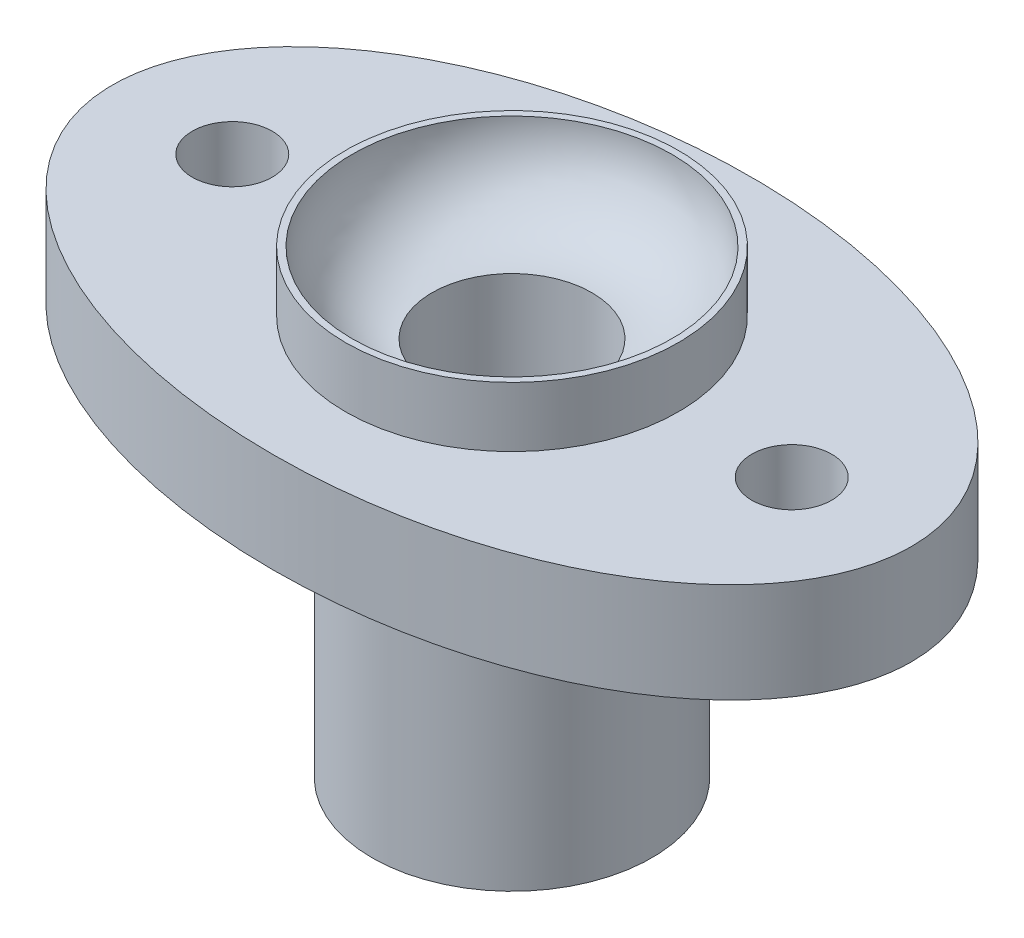
ISO-10303-21;
HEADER;
FILE_DESCRIPTION(('STEP AP214'),'2;1');
FILE_NAME('part.step','',(''),(''),'','','');
FILE_SCHEMA(('AUTOMOTIVE_DESIGN { 1 0 10303 214 1 1 1 1 }'));
ENDSEC;
DATA;
#1=APPLICATION_CONTEXT('core data for automotive mechanical design processes');
#2=APPLICATION_PROTOCOL_DEFINITION('international standard','automotive_design',2000,#1);
#3=PRODUCT_CONTEXT('',#1,'mechanical');
#4=PRODUCT('Part','Part','',(#3));
#5=PRODUCT_RELATED_PRODUCT_CATEGORY('part','',(#4));
#6=PRODUCT_DEFINITION_FORMATION('','',#4);
#7=PRODUCT_DEFINITION_CONTEXT('part definition',#1,'design');
#8=PRODUCT_DEFINITION('design','',#6,#7);
#9=PRODUCT_DEFINITION_SHAPE('','',#8);
#10=(LENGTH_UNIT() NAMED_UNIT(*) SI_UNIT(.MILLI.,.METRE.));
#11=(NAMED_UNIT(*) PLANE_ANGLE_UNIT() SI_UNIT($,.RADIAN.));
#12=(NAMED_UNIT(*) SI_UNIT($,.STERADIAN.) SOLID_ANGLE_UNIT());
#13=UNCERTAINTY_MEASURE_WITH_UNIT(LENGTH_MEASURE(1.E-05),#10,'distance_accuracy_value','');
#14=(GEOMETRIC_REPRESENTATION_CONTEXT(3) GLOBAL_UNCERTAINTY_ASSIGNED_CONTEXT((#13)) GLOBAL_UNIT_ASSIGNED_CONTEXT((#10,
#11,#12)) REPRESENTATION_CONTEXT('',''));
#15=CARTESIAN_POINT('',(0.,0.,0.));
#16=DIRECTION('',(0.,0.,1.));
#17=DIRECTION('',(1.,0.,0.));
#18=AXIS2_PLACEMENT_3D('',#15,#16,#17);
#19=CARTESIAN_POINT('',(0.,45.,0.));
#20=DIRECTION('',(0.,-1.,0.));
#21=DIRECTION('',(0.,0.,-1.));
#22=AXIS2_PLACEMENT_3D('',#19,#20,#21);
#23=CYLINDRICAL_SURFACE('',#22,21.);
#24=CARTESIAN_POINT('',(0.,45.,0.));
#25=DIRECTION('',(0.,1.,0.));
#26=DIRECTION('',(0.,0.,1.));
#27=AXIS2_PLACEMENT_3D('',#24,#25,#26);
#28=CIRCLE('',#27,21.);
#29=CARTESIAN_POINT('',(0.,45.,-21.));
#30=VERTEX_POINT('',#29);
#31=EDGE_CURVE('E10',#30,#30,#28,.T.);
#32=CARTESIAN_POINT('',(0.,0.,0.));
#33=DIRECTION('',(0.,-1.,0.));
#34=DIRECTION('',(0.,0.,-1.));
#35=AXIS2_PLACEMENT_3D('',#32,#33,#34);
#36=CIRCLE('',#35,21.);
#37=CARTESIAN_POINT('',(0.,0.,-21.));
#38=VERTEX_POINT('',#37);
#39=EDGE_CURVE('E73',#38,#38,#36,.T.);
#40=CARTESIAN_POINT('',(0.,45.,-21.));
#41=CARTESIAN_POINT('',(0.,44.53125,-21.));
#42=CARTESIAN_POINT('',(0.,44.0625,-21.));
#43=CARTESIAN_POINT('',(0.,43.125,-21.));
#44=CARTESIAN_POINT('',(0.,42.65625,-21.));
#45=CARTESIAN_POINT('',(0.,41.71875,-21.));
#46=CARTESIAN_POINT('',(0.,41.25,-21.));
#47=CARTESIAN_POINT('',(0.,40.3125,-21.));
#48=CARTESIAN_POINT('',(0.,39.84375,-21.));
#49=CARTESIAN_POINT('',(0.,38.90625,-21.));
#50=CARTESIAN_POINT('',(0.,38.4375,-21.));
#51=CARTESIAN_POINT('',(0.,37.5,-21.));
#52=CARTESIAN_POINT('',(0.,37.03125,-21.));
#53=CARTESIAN_POINT('',(0.,36.09375,-21.));
#54=CARTESIAN_POINT('',(0.,35.625,-21.));
#55=CARTESIAN_POINT('',(0.,34.6875,-21.));
#56=CARTESIAN_POINT('',(0.,34.21875,-21.));
#57=CARTESIAN_POINT('',(0.,33.28125,-21.));
#58=CARTESIAN_POINT('',(0.,32.8125,-21.));
#59=CARTESIAN_POINT('',(0.,31.875,-21.));
#60=CARTESIAN_POINT('',(0.,31.40625,-21.));
#61=CARTESIAN_POINT('',(0.,30.46875,-21.));
#62=CARTESIAN_POINT('',(0.,30.,-21.));
#63=CARTESIAN_POINT('',(0.,29.0625,-21.));
#64=CARTESIAN_POINT('',(0.,28.59375,-21.));
#65=CARTESIAN_POINT('',(0.,27.65625,-21.));
#66=CARTESIAN_POINT('',(0.,27.1875,-21.));
#67=CARTESIAN_POINT('',(0.,26.25,-21.));
#68=CARTESIAN_POINT('',(0.,25.78125,-21.));
#69=CARTESIAN_POINT('',(0.,24.84375,-21.));
#70=CARTESIAN_POINT('',(0.,24.375,-21.));
#71=CARTESIAN_POINT('',(0.,23.4375,-21.));
#72=CARTESIAN_POINT('',(0.,22.96875,-21.));
#73=CARTESIAN_POINT('',(0.,22.03125,-21.));
#74=CARTESIAN_POINT('',(0.,21.5625,-21.));
#75=CARTESIAN_POINT('',(0.,20.625,-21.));
#76=CARTESIAN_POINT('',(0.,20.15625,-21.));
#77=CARTESIAN_POINT('',(0.,19.21875,-21.));
#78=CARTESIAN_POINT('',(0.,18.75,-21.));
#79=CARTESIAN_POINT('',(0.,17.8125,-21.));
#80=CARTESIAN_POINT('',(0.,17.34375,-21.));
#81=CARTESIAN_POINT('',(0.,16.40625,-21.));
#82=CARTESIAN_POINT('',(0.,15.9375,-21.));
#83=CARTESIAN_POINT('',(0.,15.,-21.));
#84=CARTESIAN_POINT('',(0.,14.53125,-21.));
#85=CARTESIAN_POINT('',(0.,13.59375,-21.));
#86=CARTESIAN_POINT('',(0.,13.125,-21.));
#87=CARTESIAN_POINT('',(0.,12.1875,-21.));
#88=CARTESIAN_POINT('',(0.,11.71875,-21.));
#89=CARTESIAN_POINT('',(0.,10.78125,-21.));
#90=CARTESIAN_POINT('',(0.,10.3125,-21.));
#91=CARTESIAN_POINT('',(0.,9.37500000000003,-21.));
#92=CARTESIAN_POINT('',(0.,8.90625000000003,-21.));
#93=CARTESIAN_POINT('',(0.,7.96875000000003,-21.));
#94=CARTESIAN_POINT('',(0.,7.50000000000003,-21.));
#95=CARTESIAN_POINT('',(0.,6.56250000000003,-21.));
#96=CARTESIAN_POINT('',(0.,6.09375000000003,-21.));
#97=CARTESIAN_POINT('',(0.,5.15625000000003,-21.));
#98=CARTESIAN_POINT('',(0.,4.68750000000003,-21.));
#99=CARTESIAN_POINT('',(0.,3.75000000000003,-21.));
#100=CARTESIAN_POINT('',(0.,3.28125000000003,-21.));
#101=CARTESIAN_POINT('',(0.,2.34375000000003,-21.));
#102=CARTESIAN_POINT('',(0.,1.87500000000003,-21.));
#103=CARTESIAN_POINT('',(0.,0.937500000000033,-21.));
#104=CARTESIAN_POINT('',(0.,0.468750000000034,-21.));
#105=CARTESIAN_POINT('',(0.,0.,-21.));
#106=B_SPLINE_CURVE_WITH_KNOTS('',3,(#40,#41,#42,#43,#44,#45,#46,#47,#48,#49,#50,#51,#52,#53,
#54,#55,#56,#57,#58,#59,#60,#61,#62,#63,#64,#65,#66,#67,#68,#69,#70,#71,#72,#73,#74,#75,#76,#77,
#78,#79,#80,#81,#82,#83,#84,#85,#86,#87,#88,#89,#90,#91,#92,#93,#94,#95,#96,#97,#98,#99,#100,
#101,#102,#103,#104,#105),.UNSPECIFIED.,.F.,.F.,(4,2,2,2,2,2,2,2,2,2,2,2,2,2,2,2,2,2,2,2,2,2,2,
2,2,2,2,2,2,2,2,2,4),(0.,1.40625,2.8125,4.21875,5.625,7.03125,8.43749999999999,9.84375,11.25,
12.65625,14.0625,15.46875,16.875,18.28125,19.6875,21.09375,22.5,23.90625,25.3125,26.71875,
28.125,29.53125,30.9375,32.34375,33.75,35.15625,36.5625,37.96875,39.375,40.78125,42.1875,
43.59375,45.),.UNSPECIFIED.);
#107=EDGE_CURVE('BSEAM40',#30,#38,#106,.T.);
#108=ORIENTED_EDGE('',*,*,#31,.F.);
#109=ORIENTED_EDGE('',*,*,#39,.F.);
#110=ORIENTED_EDGE('',*,*,#107,.T.);
#111=ORIENTED_EDGE('',*,*,#107,.F.);
#112=EDGE_LOOP('',(#108,#110,#109,#111));
#113=FACE_BOUND('',#112,.T.);
#114=ADVANCED_FACE('F40',(#113),#23,.T.);
#115=CARTESIAN_POINT('',(0.,60.,0.));
#116=DIRECTION('',(0.,1.,0.));
#117=DIRECTION('',(1.,0.,0.));
#118=AXIS2_PLACEMENT_3D('',#115,#116,#117);
#119=ELLIPSE('',#118,60.,36.);
#120=DIRECTION('',(0.,-1.,0.));
#121=VECTOR('',#120,1.);
#122=SURFACE_OF_LINEAR_EXTRUSION('',#119,#121);
#123=CARTESIAN_POINT('',(60.,60.,0.));
#124=VERTEX_POINT('',#123);
#125=EDGE_CURVE('E42',#124,#124,#119,.T.);
#126=ORIENTED_EDGE('',*,*,#125,.F.);
#127=EDGE_LOOP('',(#126));
#128=FACE_BOUND('',#127,.T.);
#129=CARTESIAN_POINT('',(0.,45.,0.));
#130=DIRECTION('',(0.,1.,0.));
#131=DIRECTION('',(1.,0.,0.));
#132=AXIS2_PLACEMENT_3D('',#129,#130,#131);
#133=ELLIPSE('',#132,60.,36.);
#134=CARTESIAN_POINT('',(60.,45.,0.));
#135=VERTEX_POINT('',#134);
#136=EDGE_CURVE('E47',#135,#135,#133,.T.);
#137=ORIENTED_EDGE('',*,*,#136,.T.);
#138=EDGE_LOOP('',(#137));
#139=FACE_BOUND('',#138,.T.);
#140=ADVANCED_FACE('F84',(#128,#139),#122,.F.);
#141=CARTESIAN_POINT('',(0.,60.,0.));
#142=DIRECTION('',(0.,1.,0.));
#143=DIRECTION('',(0.,0.,1.));
#144=AXIS2_PLACEMENT_3D('',#141,#142,#143);
#145=PLANE('',#144);
#146=CARTESIAN_POINT('',(-42.,60.,0.));
#147=DIRECTION('',(0.,1.,0.));
#148=DIRECTION('',(0.,0.,1.));
#149=AXIS2_PLACEMENT_3D('',#146,#147,#148);
#150=CIRCLE('',#149,6.00000000000001);
#151=CARTESIAN_POINT('',(-42.,60.,6.00000000000001));
#152=VERTEX_POINT('',#151);
#153=EDGE_CURVE('E53',#152,#152,#150,.T.);
#154=ORIENTED_EDGE('',*,*,#153,.F.);
#155=EDGE_LOOP('',(#154));
#156=FACE_BOUND('',#155,.T.);
#157=CARTESIAN_POINT('',(42.,60.,0.));
#158=DIRECTION('',(0.,1.,0.));
#159=DIRECTION('',(0.,0.,1.));
#160=AXIS2_PLACEMENT_3D('',#157,#158,#159);
#161=CIRCLE('',#160,6.00000000000001);
#162=CARTESIAN_POINT('',(42.,60.,6.00000000000001));
#163=VERTEX_POINT('',#162);
#164=EDGE_CURVE('E58',#163,#163,#161,.T.);
#165=ORIENTED_EDGE('',*,*,#164,.F.);
#166=EDGE_LOOP('',(#165));
#167=FACE_BOUND('',#166,.T.);
#168=CARTESIAN_POINT('',(0.,60.,0.));
#169=DIRECTION('',(0.,1.,0.));
#170=DIRECTION('',(0.,0.,1.));
#171=AXIS2_PLACEMENT_3D('',#168,#169,#170);
#172=CIRCLE('',#171,25.);
#173=CARTESIAN_POINT('',(0.,60.,25.));
#174=VERTEX_POINT('',#173);
#175=EDGE_CURVE('E78',#174,#174,#172,.T.);
#176=ORIENTED_EDGE('',*,*,#175,.F.);
#177=EDGE_LOOP('',(#176));
#178=FACE_BOUND('',#177,.T.);
#179=ORIENTED_EDGE('',*,*,#125,.T.);
#180=EDGE_LOOP('',(#179));
#181=FACE_BOUND('',#180,.T.);
#182=ADVANCED_FACE('F87',(#156,#167,#178,#181),#145,.T.);
#183=CARTESIAN_POINT('',(0.,45.,0.));
#184=DIRECTION('',(0.,1.,0.));
#185=DIRECTION('',(0.,0.,1.));
#186=AXIS2_PLACEMENT_3D('',#183,#184,#185);
#187=PLANE('',#186);
#188=CARTESIAN_POINT('',(-42.,45.,0.));
#189=DIRECTION('',(0.,1.,0.));
#190=DIRECTION('',(0.,0.,1.));
#191=AXIS2_PLACEMENT_3D('',#188,#189,#190);
#192=CIRCLE('',#191,6.00000000000001);
#193=CARTESIAN_POINT('',(-42.,45.,6.00000000000001));
#194=VERTEX_POINT('',#193);
#195=EDGE_CURVE('E37',#194,#194,#192,.T.);
#196=ORIENTED_EDGE('',*,*,#195,.T.);
#197=EDGE_LOOP('',(#196));
#198=FACE_BOUND('',#197,.T.);
#199=CARTESIAN_POINT('',(42.,45.,0.));
#200=DIRECTION('',(0.,1.,0.));
#201=DIRECTION('',(0.,0.,1.));
#202=AXIS2_PLACEMENT_3D('',#199,#200,#201);
#203=CIRCLE('',#202,6.00000000000001);
#204=CARTESIAN_POINT('',(42.,45.,6.00000000000001));
#205=VERTEX_POINT('',#204);
#206=EDGE_CURVE('E55',#205,#205,#203,.T.);
#207=ORIENTED_EDGE('',*,*,#206,.T.);
#208=EDGE_LOOP('',(#207));
#209=FACE_BOUND('',#208,.T.);
#210=ORIENTED_EDGE('',*,*,#31,.T.);
#211=EDGE_LOOP('',(#210));
#212=FACE_BOUND('',#211,.T.);
#213=ORIENTED_EDGE('',*,*,#136,.F.);
#214=EDGE_LOOP('',(#213));
#215=FACE_BOUND('',#214,.T.);
#216=ADVANCED_FACE('F90',(#198,#209,#212,#215),#187,.F.);
#217=CARTESIAN_POINT('',(0.,69.,0.));
#218=DIRECTION('',(0.,-1.,0.));
#219=DIRECTION('',(0.,0.,-1.));
#220=AXIS2_PLACEMENT_3D('',#217,#218,#219);
#221=CYLINDRICAL_SURFACE('',#220,25.);
#222=CARTESIAN_POINT('',(0.,69.,0.));
#223=DIRECTION('',(0.,1.,0.));
#224=DIRECTION('',(0.,0.,1.));
#225=AXIS2_PLACEMENT_3D('',#222,#223,#224);
#226=CIRCLE('',#225,25.);
#227=CARTESIAN_POINT('',(0.,69.,25.));
#228=VERTEX_POINT('',#227);
#229=EDGE_CURVE('E79',#228,#228,#226,.T.);
#230=ORIENTED_EDGE('',*,*,#229,.F.);
#231=EDGE_LOOP('',(#230));
#232=FACE_BOUND('',#231,.T.);
#233=ORIENTED_EDGE('',*,*,#175,.T.);
#234=EDGE_LOOP('',(#233));
#235=FACE_BOUND('',#234,.T.);
#236=ADVANCED_FACE('F95',(#232,#235),#221,.T.);
#237=CARTESIAN_POINT('',(0.,69.,0.));
#238=DIRECTION('',(0.,1.,0.));
#239=DIRECTION('',(0.,0.,1.));
#240=AXIS2_PLACEMENT_3D('',#237,#238,#239);
#241=PLANE('',#240);
#242=CARTESIAN_POINT('',(0.,69.,0.));
#243=DIRECTION('',(0.,-1.,0.));
#244=DIRECTION('',(0.,0.,-1.));
#245=AXIS2_PLACEMENT_3D('',#242,#243,#244);
#246=CIRCLE('',#245,24.);
#247=CARTESIAN_POINT('',(0.,69.,-24.));
#248=VERTEX_POINT('',#247);
#249=EDGE_CURVE('E59',#248,#248,#246,.T.);
#250=ORIENTED_EDGE('',*,*,#249,.T.);
#251=EDGE_LOOP('',(#250));
#252=FACE_BOUND('',#251,.T.);
#253=ORIENTED_EDGE('',*,*,#229,.T.);
#254=EDGE_LOOP('',(#253));
#255=FACE_BOUND('',#254,.T.);
#256=ADVANCED_FACE('F97',(#252,#255),#241,.T.);
#257=CARTESIAN_POINT('',(0.,0.,0.));
#258=DIRECTION('',(0.,-1.,0.));
#259=DIRECTION('',(0.,0.,-1.));
#260=AXIS2_PLACEMENT_3D('',#257,#258,#259);
#261=CONICAL_SURFACE('',#260,21.,1.30899693899575);
#262=CARTESIAN_POINT('',(0.,2.41154273188007,0.));
#263=DIRECTION('',(0.,-1.,0.));
#264=DIRECTION('',(0.,0.,-1.));
#265=AXIS2_PLACEMENT_3D('',#262,#263,#264);
#266=CIRCLE('',#265,12.);
#267=CARTESIAN_POINT('',(0.,2.41154273188007,-12.));
#268=VERTEX_POINT('',#267);
#269=EDGE_CURVE('E75',#268,#268,#266,.T.);
#270=ORIENTED_EDGE('',*,*,#269,.F.);
#271=EDGE_LOOP('',(#270));
#272=FACE_BOUND('',#271,.T.);
#273=ORIENTED_EDGE('',*,*,#39,.T.);
#274=EDGE_LOOP('',(#273));
#275=FACE_BOUND('',#274,.T.);
#276=ADVANCED_FACE('F103',(#272,#275),#261,.F.);
#277=CARTESIAN_POINT('',(0.,0.,0.));
#278=DIRECTION('',(0.,-1.,0.));
#279=DIRECTION('',(0.,0.,-1.));
#280=AXIS2_PLACEMENT_3D('',#277,#278,#279);
#281=CYLINDRICAL_SURFACE('',#280,12.);
#282=CARTESIAN_POINT('',(0.,57.,0.));
#283=DIRECTION('',(0.,-1.,0.));
#284=DIRECTION('',(0.,0.,-1.));
#285=AXIS2_PLACEMENT_3D('',#282,#283,#284);
#286=CIRCLE('',#285,12.);
#287=CARTESIAN_POINT('',(0.,57.,-12.));
#288=VERTEX_POINT('',#287);
#289=EDGE_CURVE('E69',#288,#288,#286,.T.);
#290=ORIENTED_EDGE('',*,*,#289,.F.);
#291=EDGE_LOOP('',(#290));
#292=FACE_BOUND('',#291,.T.);
#293=ORIENTED_EDGE('',*,*,#269,.T.);
#294=EDGE_LOOP('',(#293));
#295=FACE_BOUND('',#294,.T.);
#296=ADVANCED_FACE('F110',(#292,#295),#281,.F.);
#297=CARTESIAN_POINT('',(0.,69.,0.));
#298=DIRECTION('',(0.,-1.,0.));
#299=DIRECTION('',(0.,0.,-1.));
#300=AXIS2_PLACEMENT_3D('',#297,#298,#299);
#301=TOROIDAL_SURFACE('',#300,12.,12.);
#302=ORIENTED_EDGE('',*,*,#249,.F.);
#303=EDGE_LOOP('',(#302));
#304=FACE_BOUND('',#303,.T.);
#305=ORIENTED_EDGE('',*,*,#289,.T.);
#306=EDGE_LOOP('',(#305));
#307=FACE_BOUND('',#306,.T.);
#308=ADVANCED_FACE('F112',(#304,#307),#301,.F.);
#309=CARTESIAN_POINT('',(42.,41.,0.));
#310=DIRECTION('',(0.,1.,0.));
#311=DIRECTION('',(0.,0.,1.));
#312=AXIS2_PLACEMENT_3D('',#309,#310,#311);
#313=CYLINDRICAL_SURFACE('',#312,6.00000000000001);
#314=ORIENTED_EDGE('',*,*,#164,.T.);
#315=EDGE_LOOP('',(#314));
#316=FACE_BOUND('',#315,.T.);
#317=ORIENTED_EDGE('',*,*,#206,.F.);
#318=EDGE_LOOP('',(#317));
#319=FACE_BOUND('',#318,.T.);
#320=ADVANCED_FACE('F113',(#316,#319),#313,.F.);
#321=CARTESIAN_POINT('',(-42.,41.,0.));
#322=DIRECTION('',(0.,1.,0.));
#323=DIRECTION('',(0.,0.,1.));
#324=AXIS2_PLACEMENT_3D('',#321,#322,#323);
#325=CYLINDRICAL_SURFACE('',#324,6.00000000000001);
#326=ORIENTED_EDGE('',*,*,#153,.T.);
#327=EDGE_LOOP('',(#326));
#328=FACE_BOUND('',#327,.T.);
#329=ORIENTED_EDGE('',*,*,#195,.F.);
#330=EDGE_LOOP('',(#329));
#331=FACE_BOUND('',#330,.T.);
#332=ADVANCED_FACE('F119',(#328,#331),#325,.F.);
#333=CLOSED_SHELL('',(#114,#140,#182,#216,#236,#256,#276,#296,#308,#320,#332));
#334=MANIFOLD_SOLID_BREP('B2',#333);
#335=ADVANCED_BREP_SHAPE_REPRESENTATION('',(#18,#334),#14);
#336=SHAPE_DEFINITION_REPRESENTATION(#9,#335);
ENDSEC;
END-ISO-10303-21;
